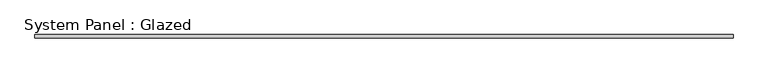
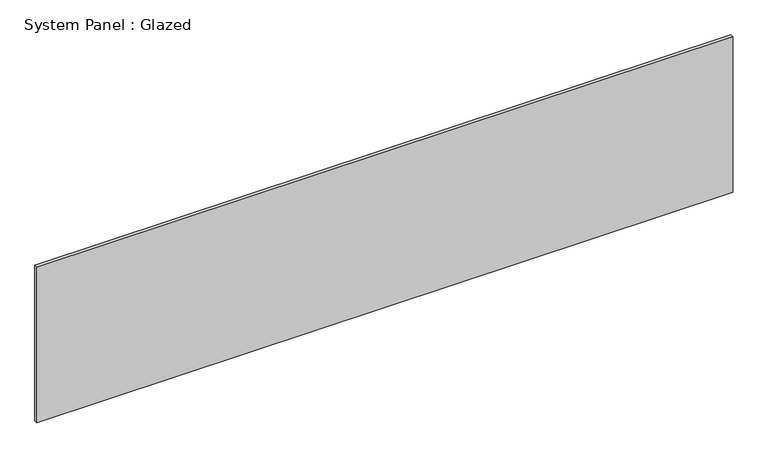
"""IFC4 building model written with IfcOpenShell, lengths in millimetres: plate geometry, System Panel : Glazed."""

from ifc_helpers import new_model, si_unit, origin, origin_with_axes, place, context, project, spatial, polyline, outline, extrude, source, transform, mapped, element, save


def system_panel_glazed_605ab5bb(model_context):
    return source(origin(), model_context, "Body", "SweptSolid", [
        extrude(outline(polyline([(2586.7052025, 19.05), (-2586.7052025, 19.05), (-2586.7052025, 44.45), (2586.7052025, 44.45), (2586.7052025, 19.05)])), origin_with_axes(), (0.0, 0.0, 1.0), 1219.2),
    ])


if __name__ == "__main__":
    model = new_model("IFC4")
    model_context = context("Model", 3, world=origin())
    ifc_project = project(units=[si_unit("LENGTHUNIT", "METRE", prefix="MILLI")], contexts=[model_context])
    site = spatial("IfcSite", under=ifc_project)
    building = spatial("IfcBuilding", under=site)
    placement = place(None, origin())
    system_panel_glazed_shape = system_panel_glazed_605ab5bb(model_context)
    element("IfcPlate", 1, ObjectType="System Panel : Glazed", at=placement, inside=building, context=model_context, shape_type="MappedRepresentation", body=[
        mapped(system_panel_glazed_shape, transform((0.0, 0.0, 0.0), x_axis=(1.0, 0.0, 0.0), y_axis=(0.0, 1.0, 0.0), z_axis=(0.0, 0.0, 1.0))),
    ])
    save(model, "model.ifc")

# Revit data of these elements
# Type "System Panel : Glazed"
#   Construction Type Id = "GSP4R"
#   Analytic Construction = "1/8 in Pilkington single glazing"
#   Visual Light Transmittance = 0.9
#   Solar Heat Gain Coefficient = 0.86
#   Heat Transfer Coefficient (U) = 1.18115 BTU/(h·ft²·°F)
# Element 1 (IfcPlate, "System Panel : Glazed")
#   Materials on its faces: "Glass"
# Materials
#   "Glass": class "Glass", colour RGB 0 128 192, transparency 0.75, Description = "Soda Lime Glass", Cost = 0
